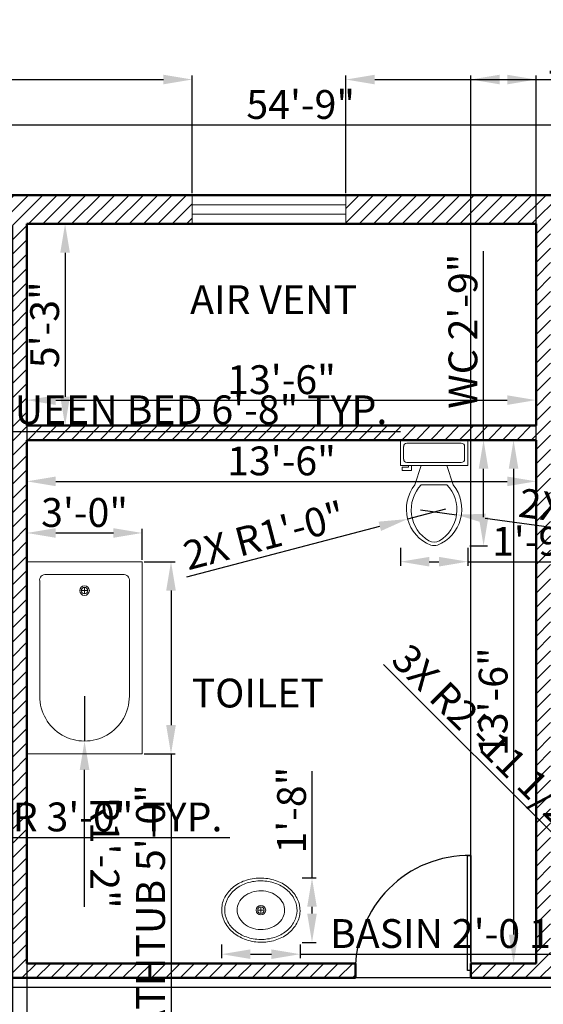
# Model space of a CAD drawing. Units: inches. Extents: x 61993 to 62774, y 55335 to 55871.
# Tile 4 of 6: x 62310 to 62474, y 55563 to 55871. Entities that reach past the tile are written whole.
import ezdxf

# ---------------------------------------------------------------- set-up
doc = ezdxf.new("R2010")
doc.units = ezdxf.units.IN
for name, color, linetype, lineweight in [('A-ANNO-DIMS', 2, 'Continuous', 18), ('A-AREA-IDEN', 7, 'Continuous', 25), ('A-DOOR', 3, 'Continuous', 25), ('A-FLOR-FIXT', 9, 'Continuous', 18), ('A-GLAZ', 4, 'Continuous', 18), ('A-WALL', 7, 'Continuous', 50)]:
    doc.layers.add(name, color=color, linetype=linetype, lineweight=lineweight)
doc.layers.add('A-WALL-PATT', color=40, linetype='Continuous', lineweight=13, true_color=0xf8d731)
doc.styles.get("Standard").update_dxf_attribs({"font": 'arial.ttf'})
doc.dimstyles.new('ISO-25', dxfattribs={"dimtxt": 9, "dimasz": 9, "dimexe": 1.25, "dimexo": 0.625, "dimtad": 1, "dimdec": 1, "dimrnd": 9, "dimlunit": 3, "dimtxsty": 'Standard', "dimcen": 2.5, "dimadec": 0, "dimazin": 0, "dimtfac": 1, "dimtdec": 1, "dimtmove": 0, "dimatfit": 3, "dimfxl": 1, "dimarcsym": 0})

# ---------------------------------------------------------------- blocks, each defined once
blk = doc.blocks.new('*D3')
at = {"layer": 'A-ANNO-DIMS', "color": 0, "lineweight": -2, "transparency": 16777216}
for p, q in [((62312.69, 55744.58), (62312.69, 55753.17)), ((62471.69, 55744.58), (62471.69, 55753.17)), ((62321.69, 55751.92), (62462.69, 55751.92))]:
    blk.add_line(p, q, dxfattribs=at)
at = {"layer": 'A-ANNO-DIMS', "color": 0, "transparency": 16777216}
for points in [[(62321.69, 55753.42), (62321.69, 55750.42), (62312.69, 55751.92)], [(62462.69, 55753.42), (62462.69, 55750.42), (62471.69, 55751.92)]]:
    blk.add_solid(points, dxfattribs=at)
at = {"layer": 'Defpoints', "color": 0, "transparency": 16777216}
for p in [(62471.69, 55751.92), (62312.69, 55743.96), (62471.69, 55743.96)]:
    blk.add_point(p, dxfattribs=at)
at = {"layer": 'A-ANNO-DIMS', "color": 0, "transparency": 16777216, "insert": (62392.19, 55757.14), "char_height": 9, "attachment_point": 5}
blk.add_mtext('13\'-6"', dxfattribs=at)
blk = doc.blocks.new('*D4')
at = {"layer": 'A-ANNO-DIMS', "color": 0, "lineweight": -2, "transparency": 16777216}
for p, q in [((62313.32, 55806.96), (62325.87, 55806.96)), ((62324.62, 55797.96), (62324.62, 55752.96)), ((62313.32, 55743.96), (62325.87, 55743.96))]:
    blk.add_line(p, q, dxfattribs=at)
at = {"layer": 'A-ANNO-DIMS', "color": 0, "transparency": 16777216}
for points in [[(62323.12, 55797.96), (62326.12, 55797.96), (62324.62, 55806.96)], [(62323.12, 55752.96), (62326.12, 55752.96), (62324.62, 55743.96)]]:
    blk.add_solid(points, dxfattribs=at)
at = {"layer": 'Defpoints', "color": 0, "transparency": 16777216}
for p in [(62312.69, 55806.96), (62312.69, 55743.96), (62324.62, 55743.96)]:
    blk.add_point(p, dxfattribs=at)
at = {"layer": 'A-ANNO-DIMS', "color": 0, "transparency": 16777216, "insert": (62319.39, 55775.46), "char_height": 9, "attachment_point": 5, "rotation": 90}
blk.add_mtext('5\'-3"', dxfattribs=at)
blk = doc.blocks.new('*D5')
at = {"layer": 'A-ANNO-DIMS', "color": 0, "lineweight": -2, "transparency": 16777216}
for p, q in [((62471.07, 55739.46), (62463.41, 55739.46)), ((62464.66, 55730.46), (62464.66, 55584.96)), ((62471.07, 55575.96), (62463.41, 55575.96))]:
    blk.add_line(p, q, dxfattribs=at)
at = {"layer": 'A-ANNO-DIMS', "color": 0, "transparency": 16777216}
for points in [[(62463.16, 55730.46), (62466.16, 55730.46), (62464.66, 55739.46)], [(62463.16, 55584.96), (62466.16, 55584.96), (62464.66, 55575.96)]]:
    blk.add_solid(points, dxfattribs=at)
at = {"layer": 'Defpoints', "color": 0, "transparency": 16777216}
for p in [(62471.69, 55739.46), (62464.66, 55575.96), (62471.69, 55575.96)]:
    blk.add_point(p, dxfattribs=at)
at = {"layer": 'A-ANNO-DIMS', "color": 0, "transparency": 16777216, "insert": (62459.44, 55657.71), "char_height": 9, "attachment_point": 5, "rotation": 90}
blk.add_mtext('13\'-6"', dxfattribs=at)
blk = doc.blocks.new('*D6')
at = {"layer": 'A-ANNO-DIMS', "color": 0, "lineweight": -2, "transparency": 16777216}
for p, q in [((62312.69, 55738.83), (62312.69, 55725.29)), ((62471.69, 55738.83), (62471.69, 55725.29)), ((62321.69, 55726.54), (62462.69, 55726.54))]:
    blk.add_line(p, q, dxfattribs=at)
at = {"layer": 'A-ANNO-DIMS', "color": 0, "transparency": 16777216}
for points in [[(62321.69, 55728.04), (62321.69, 55725.04), (62312.69, 55726.54)], [(62462.69, 55728.04), (62462.69, 55725.04), (62471.69, 55726.54)]]:
    blk.add_solid(points, dxfattribs=at)
at = {"layer": 'Defpoints', "color": 0, "transparency": 16777216}
for p in [(62312.69, 55739.46), (62471.69, 55739.46), (62471.69, 55726.54)]:
    blk.add_point(p, dxfattribs=at)
at = {"layer": 'A-ANNO-DIMS', "color": 0, "transparency": 16777216, "insert": (62392.19, 55731.76), "char_height": 9, "attachment_point": 5}
blk.add_mtext('13\'-6"', dxfattribs=at)
blk = doc.blocks.new('Toilet - top')
for p, q in [((9.5, -6), (9.5, -2)), ((-10, -8.5), (-8, -8.5)), ((-10, -9.5), (-10, -8.5)), ((-8, -8.5), (-8, -8)), ((-7, -8), (-7, -9.5)), ((-4, -8), (-6, -14)), ((4, -8), (6, -14)), ((-7, -9.5), (-10, -9.5)), ((4, -14), (-4, -14))]:
    blk.add_line(p, q)
blk.add_lwpolyline([(10.5, -8), (10.5, 0), (-10.5, 0), (-10.5, -8)], close=True)
for points in [[(-9.5, -2), (-9.5, -6)], [(8.5, -1), (-8.5, -1)], [(-8.5, -7), (8.5, -7)]]:
    blk.add_lwpolyline(points)
for centre, radius, start, end in [((-8.62, -1.88), 0.884, 81.8699, 188.1301), ((8.62, -1.88), 0.884, 351.8699, 98.1301), ((-8.62, -6.12), 0.884, 171.8699, 278.1301), ((8.62, -6.12), 0.884, 261.8699, 8.1301), ((3.52, -21.58), 12.17, 141.4691, 247.9714), ((4.2, -21.82), 11.33, 136.3677, 238.9468), ((-3.52, -21.58), 12.17, 292.0284, 38.5307), ((-4.2, -21.82), 11.33, 301.053, 43.6321), ((0, -27.88), 4, 245.7318, 294.2682), ((0, -29), 4, 254.8605, 285.1395)]:
    blk.add_arc(centre, radius, start, end)
blk = doc.blocks.new('Sink - Oval top')
for p, q in [((-1, 0), (1, 0)), ((0, 1), (0, -1))]:
    blk.add_line(p, q)
for points in [[(-12.23, 0.39, 0.117634), (-11.46, -3.36, 0.104469), (-8.88, -6.8, 0.090016), (-5.08, -9.07, 0.08192), (-0.32, -10.02, 0.08192), (4.49, -9.38, 0.090016), (8.42, -7.36, 0.104469), (11.22, -4.09, 0.117634), (12.23, -0.39, 0.117634), (11.46, 3.36, 0.104469), (8.88, 6.8, 0.090016), (5.08, 9.07, 0.08192), (0.32, 10.02, 0.08192), (-4.49, 9.38, 0.090016), (-8.42, 7.36, 0.104469), (-11.22, 4.09, 0.117634)], [(-11.29, 0.16, 0.118622), (-10.52, -3.25, 0.104678), (-8.07, -6.36, 0.089562), (-4.54, -8.37, 0.081185), (-0.13, -9.15, 0.081185), (4.3, -8.49, 0.089562), (7.89, -6.58, 0.104678), (10.42, -3.55, 0.118622), (11.29, -0.16, 0.118622), (10.52, 3.25, 0.104678), (8.07, 6.36, 0.089562), (4.54, 8.37, 0.081185), (0.13, 9.15, 0.081185), (-4.3, 8.49, 0.089562), (-7.89, 6.58, 0.104678), (-10.42, 3.55, 0.118622)], [(-7.42, 0.08, 0.118283), (-6.91, -2.17, 0.104607), (-5.29, -4.21, 0.089718), (-2.97, -5.53, 0.081436), (-0.07, -6.04, 0.081436), (2.84, -5.59, 0.089718), (5.2, -4.33, 0.104607), (6.86, -2.32, 0.118283), (7.42, -0.08, 0.118283), (6.91, 2.17, 0.104607), (5.29, 4.21, 0.089718), (2.97, 5.53, 0.081436), (0.07, 6.04, 0.081436), (-2.84, 5.59, 0.089718), (-5.2, 4.33, 0.104607), (-6.86, 2.32, 0.118283)]]:
    blk.add_lwpolyline(points, format="xyb", close=True)
for radius in [1.5, 1]:
    blk.add_circle((0, 0), radius)
blk = doc.blocks.new('Bath Tub - 26 x 60 in.')
for p, q in [((8, -18), (10, -18)), ((9, -17), (9, -19))]:
    blk.add_line(p, q)
blk.add_lwpolyline([(0, -36), (0, 0), (60, 0), (60, -36)], close=True)
for points in [[(4, -30), (4, -6)], [(6, -4), (42, -4)], [(42, -32), (6, -32)]]:
    blk.add_lwpolyline(points)
for radius in [1.5, 1]:
    blk.add_circle((9, -18), radius)
for centre, radius, start, end in [((5.75, -5.75), 1.77, 81.8699, 188.1301), ((42, -18), 14, 270, 90), ((5.75, -30.25), 1.77, 171.8699, 278.1301)]:
    blk.add_arc(centre, radius, start, end)
blk = doc.blocks.new('*D24')
at = {"layer": 'A-ANNO-DIMS', "color": 0, "lineweight": -2, "transparency": 16777216}
for p, q in [((62068.19, 55816.58), (62068.19, 55839.13)), ((62728.19, 55816.58), (62728.19, 55839.13)), ((62077.19, 55837.88), (62719.19, 55837.88))]:
    blk.add_line(p, q, dxfattribs=at)
at = {"layer": 'A-ANNO-DIMS', "color": 0, "transparency": 16777216}
for points in [[(62077.19, 55839.38), (62077.19, 55836.38), (62068.19, 55837.88)], [(62719.19, 55839.38), (62719.19, 55836.38), (62728.19, 55837.88)]]:
    blk.add_solid(points, dxfattribs=at)
at = {"layer": 'Defpoints', "color": 0, "transparency": 16777216}
for p in [(62728.19, 55837.88), (62068.19, 55815.96), (62728.19, 55815.96)]:
    blk.add_point(p, dxfattribs=at)
at = {"layer": 'A-ANNO-DIMS', "color": 0, "transparency": 16777216, "insert": (62398.19, 55843.1), "char_height": 9, "attachment_point": 5}
blk.add_mtext('54\'-9"', dxfattribs=at)
blk = doc.blocks.new('WIN-48IN')
for p, q in [((0, 9), (0, 0)), ((48, 9), (48, 0)), ((48, 6), (0, 6)), ((48, 3), (0, 3))]:
    blk.add_line(p, q)
blk = doc.blocks.new('DOOR-SINGLE-36IN')
for p, q in [((35, 0), (35, 36)), ((35, 36), (36, 36)), ((36, 36), (36, 2.25)), ((36, 0), (35, 0))]:
    blk.add_line(p, q)
blk.add_arc((35.5, 0.5), 35.5, 89.1931, 180.8069)
blk = doc.blocks.new('*D34')
at = {"layer": 'A-ANNO-DIMS', "color": 0, "lineweight": -2, "transparency": 16777216}
for p, q in [((62234.09, 55610.47), (62234.09, 55616.51)), ((62243.09, 55615.26), (62261.23, 55615.26)), ((62270.23, 55610.47), (62270.23, 55616.51)), ((62270.23, 55615.26), (62376.1, 55615.26))]:
    blk.add_line(p, q, dxfattribs=at)
at = {"layer": 'A-ANNO-DIMS', "color": 0, "transparency": 16777216}
for points in [[(62243.09, 55616.76), (62243.09, 55613.76), (62234.09, 55615.26)], [(62261.23, 55616.76), (62261.23, 55613.76), (62270.23, 55615.26)]]:
    blk.add_solid(points, dxfattribs=at)
at = {"layer": 'Defpoints', "color": 0, "transparency": 16777216}
for p in [(62270.23, 55615.26), (62234.09, 55609.84), (62270.23, 55609.84)]:
    blk.add_point(p, dxfattribs=at)
at = {"layer": 'A-ANNO-DIMS', "color": 0, "transparency": 16777216, "insert": (62327.67, 55620.55), "char_height": 9, "attachment_point": 5}
blk.add_mtext('DOOR 3\'-0" TYP.', dxfattribs=at)
blk = doc.blocks.new('*D38')
at = {"layer": 'A-ANNO-DIMS', "color": 0, "lineweight": -2, "transparency": 16777216}
for p, q in [((62206.68, 55730.79), (62206.68, 55743.42)), ((62286.68, 55730.79), (62286.68, 55743.42)), ((62215.68, 55742.17), (62277.68, 55742.17)), ((62286.68, 55742.17), (62429.32, 55742.17))]:
    blk.add_line(p, q, dxfattribs=at)
at = {"layer": 'A-ANNO-DIMS', "color": 0, "transparency": 16777216}
for points in [[(62215.68, 55743.67), (62215.68, 55740.67), (62206.68, 55742.17)], [(62277.68, 55743.67), (62277.68, 55740.67), (62286.68, 55742.17)]]:
    blk.add_solid(points, dxfattribs=at)
at = {"layer": 'Defpoints', "color": 0, "transparency": 16777216}
for p in [(62286.68, 55742.17), (62206.68, 55730.17), (62286.68, 55730.17)]:
    blk.add_point(p, dxfattribs=at)
at = {"layer": 'A-ANNO-DIMS', "color": 0, "transparency": 16777216, "insert": (62362.5, 55747.72), "char_height": 9, "attachment_point": 5}
blk.add_mtext('QUEEN BED 6\'-8" TYP.', dxfattribs=at)
blk = doc.blocks.new('*D44')
at = {"layer": 'A-ANNO-DIMS', "color": 0, "lineweight": -2, "transparency": 16777216}
for p, q in [((62455.29, 55739.46), (62455.29, 55798.44)), ((62450.96, 55739.46), (62456.54, 55739.46)), ((62455.29, 55715.41), (62455.29, 55730.46)), ((62450.96, 55706.41), (62456.54, 55706.41))]:
    blk.add_line(p, q, dxfattribs=at)
at = {"layer": 'A-ANNO-DIMS', "color": 0, "transparency": 16777216}
for points in [[(62453.79, 55730.46), (62456.79, 55730.46), (62455.29, 55739.46)], [(62453.79, 55715.41), (62456.79, 55715.41), (62455.29, 55706.41)]]:
    blk.add_solid(points, dxfattribs=at)
at = {"layer": 'Defpoints', "color": 0, "transparency": 16777216}
for p in [(62450.34, 55739.46), (62455.29, 55739.46), (62450.34, 55706.41)]:
    blk.add_point(p, dxfattribs=at)
at = {"layer": 'A-ANNO-DIMS', "color": 0, "transparency": 16777216, "insert": (62450.01, 55773.45), "char_height": 9, "attachment_point": 5, "rotation": 90}
blk.add_mtext('WC 2\'-9"', dxfattribs=at)
blk = doc.blocks.new('*D45')
at = {"layer": 'A-ANNO-DIMS', "color": 0, "lineweight": -2, "transparency": 16777216}
for p, q in [((62429.34, 55705.79), (62429.34, 55700.2)), ((62450.34, 55705.79), (62450.34, 55700.2)), ((62438.34, 55701.45), (62441.34, 55701.45)), ((62450.34, 55701.45), (62483.66, 55701.45))]:
    blk.add_line(p, q, dxfattribs=at)
at = {"layer": 'A-ANNO-DIMS', "color": 0, "transparency": 16777216}
for points in [[(62438.34, 55702.95), (62438.34, 55699.95), (62429.34, 55701.45)], [(62441.34, 55702.95), (62441.34, 55699.95), (62450.34, 55701.45)]]:
    blk.add_solid(points, dxfattribs=at)
at = {"layer": 'Defpoints', "color": 0, "transparency": 16777216}
for p in [(62429.34, 55706.41), (62450.34, 55706.41), (62450.34, 55701.45)]:
    blk.add_point(p, dxfattribs=at)
at = {"layer": 'A-ANNO-DIMS', "color": 0, "transparency": 16777216, "insert": (62471.5, 55706.67), "char_height": 9, "attachment_point": 5}
blk.add_mtext('1\'-9"', dxfattribs=at)
blk = doc.blocks.new('*D46')
at = {"layer": 'A-ANNO-DIMS', "color": 0, "lineweight": -2, "transparency": 16777216}
for p, q in [((62373.49, 55581.91), (62373.49, 55577.6)), ((62398.04, 55581.91), (62398.04, 55577.6)), ((62382.49, 55578.85), (62389.04, 55578.85)), ((62398.04, 55578.85), (62494.01, 55578.85))]:
    blk.add_line(p, q, dxfattribs=at)
at = {"layer": 'A-ANNO-DIMS', "color": 0, "transparency": 16777216}
for points in [[(62382.49, 55580.35), (62382.49, 55577.35), (62373.49, 55578.85)], [(62389.04, 55580.35), (62389.04, 55577.35), (62398.04, 55578.85)]]:
    blk.add_solid(points, dxfattribs=at)
at = {"layer": 'Defpoints', "color": 0, "transparency": 16777216}
for p in [(62373.49, 55582.54), (62398.04, 55582.54), (62398.04, 55578.85)]:
    blk.add_point(p, dxfattribs=at)
at = {"layer": 'A-ANNO-DIMS', "color": 0, "transparency": 16777216, "insert": (62450.52, 55584.13), "char_height": 9, "attachment_point": 5}
blk.add_mtext('BASIN 2\'-0 1/2"', dxfattribs=at)
blk = doc.blocks.new('*D47')
at = {"layer": 'A-ANNO-DIMS', "color": 0, "lineweight": -2, "transparency": 16777216}
for p, q in [((62401.72, 55602.67), (62401.72, 55636)), ((62398.66, 55602.67), (62402.97, 55602.67)), ((62401.72, 55591.54), (62401.72, 55593.67)), ((62398.66, 55582.54), (62402.97, 55582.54))]:
    blk.add_line(p, q, dxfattribs=at)
at = {"layer": 'A-ANNO-DIMS', "color": 0, "transparency": 16777216}
for points in [[(62400.22, 55593.67), (62403.22, 55593.67), (62401.72, 55602.67)], [(62400.22, 55591.54), (62403.22, 55591.54), (62401.72, 55582.54)]]:
    blk.add_solid(points, dxfattribs=at)
at = {"layer": 'Defpoints', "color": 0, "transparency": 16777216}
for p in [(62398.04, 55602.67), (62401.72, 55602.67), (62398.04, 55582.54)]:
    blk.add_point(p, dxfattribs=at)
at = {"layer": 'A-ANNO-DIMS', "color": 0, "transparency": 16777216, "insert": (62396.5, 55623.84), "char_height": 9, "attachment_point": 5, "rotation": 90}
blk.add_mtext('1\'-8"', dxfattribs=at)
blk = doc.blocks.new('*D48')
at = {"layer": 'A-ANNO-DIMS', "color": 0, "lineweight": -2, "transparency": 16777216}
for p, q in [((62349.32, 55701.42), (62358.94, 55701.42)), ((62357.69, 55692.42), (62357.69, 55650.42)), ((62349.32, 55641.42), (62358.94, 55641.42)), ((62357.69, 55641.42), (62357.69, 55545.48))]:
    blk.add_line(p, q, dxfattribs=at)
at = {"layer": 'A-ANNO-DIMS', "color": 0, "transparency": 16777216}
for points in [[(62356.19, 55692.42), (62359.19, 55692.42), (62357.69, 55701.42)], [(62356.19, 55650.42), (62359.19, 55650.42), (62357.69, 55641.42)]]:
    blk.add_solid(points, dxfattribs=at)
at = {"layer": 'Defpoints', "color": 0, "transparency": 16777216}
for p in [(62348.69, 55701.42), (62348.69, 55641.42), (62357.69, 55641.42)]:
    blk.add_point(p, dxfattribs=at)
at = {"layer": 'A-ANNO-DIMS', "color": 0, "transparency": 16777216, "insert": (62352.47, 55588.95), "char_height": 9, "attachment_point": 5, "rotation": 90}
blk.add_mtext('BATHTUB 5\'-0"', dxfattribs=at)
blk = doc.blocks.new('*D49')
at = {"layer": 'A-ANNO-DIMS', "color": 0, "lineweight": -2, "transparency": 16777216}
for p, q in [((62312.69, 55702.05), (62312.69, 55711.67)), ((62321.69, 55710.42), (62339.69, 55710.42)), ((62348.69, 55702.05), (62348.69, 55711.67))]:
    blk.add_line(p, q, dxfattribs=at)
at = {"layer": 'A-ANNO-DIMS', "color": 0, "transparency": 16777216}
for points in [[(62321.69, 55711.92), (62321.69, 55708.92), (62312.69, 55710.42)], [(62339.69, 55711.92), (62339.69, 55708.92), (62348.69, 55710.42)]]:
    blk.add_solid(points, dxfattribs=at)
at = {"layer": 'Defpoints', "color": 0, "transparency": 16777216}
for p in [(62348.69, 55710.42), (62312.69, 55701.42), (62348.69, 55701.42)]:
    blk.add_point(p, dxfattribs=at)
at = {"layer": 'A-ANNO-DIMS', "color": 0, "transparency": 16777216, "insert": (62330.69, 55715.65), "char_height": 9, "attachment_point": 5}
blk.add_mtext('3\'-0"', dxfattribs=at)
blk = doc.blocks.new('*D65')
at = {"layer": 'A-ANNO-DIMS', "color": 0, "lineweight": -2, "transparency": 16777216}
for p, q in [((62186.51, 55816.58), (62186.51, 55853.31)), ((62195.51, 55852.06), (62355.31, 55852.06)), ((62364.31, 55816.58), (62364.31, 55853.31))]:
    blk.add_line(p, q, dxfattribs=at)
at = {"layer": 'A-ANNO-DIMS', "color": 0, "transparency": 16777216}
for points in [[(62195.51, 55853.56), (62195.51, 55850.56), (62186.51, 55852.06)], [(62355.31, 55853.56), (62355.31, 55850.56), (62364.31, 55852.06)]]:
    blk.add_solid(points, dxfattribs=at)
at = {"layer": 'Defpoints', "color": 0, "transparency": 16777216}
for p in [(62364.31, 55852.06), (62186.51, 55815.96), (62364.31, 55815.96)]:
    blk.add_point(p, dxfattribs=at)
at = {"layer": 'A-ANNO-DIMS', "color": 0, "transparency": 16777216, "insert": (62275.41, 55857.28), "char_height": 9, "attachment_point": 5}
blk.add_mtext('14\'-10"', dxfattribs=at)
blk = doc.blocks.new('*D66')
at = {"layer": 'A-ANNO-DIMS', "color": 0, "lineweight": -2, "transparency": 16777216}
for p, q in [((62412.31, 55816.58), (62412.31, 55853.31)), ((62421.31, 55852.06), (62569.07, 55852.06)), ((62578.07, 55816.58), (62578.07, 55853.31))]:
    blk.add_line(p, q, dxfattribs=at)
at = {"layer": 'A-ANNO-DIMS', "color": 0, "transparency": 16777216}
for points in [[(62421.31, 55853.56), (62421.31, 55850.56), (62412.31, 55852.06)], [(62569.07, 55853.56), (62569.07, 55850.56), (62578.07, 55852.06)]]:
    blk.add_solid(points, dxfattribs=at)
at = {"layer": 'Defpoints', "color": 0, "transparency": 16777216}
for p in [(62578.07, 55852.06), (62412.31, 55815.96), (62578.07, 55815.96)]:
    blk.add_point(p, dxfattribs=at)
at = {"layer": 'A-ANNO-DIMS', "color": 0, "transparency": 16777216, "insert": (62495.19, 55857.28), "char_height": 9, "attachment_point": 5}
blk.add_mtext('13\'-10"', dxfattribs=at)
blk = doc.blocks.new('*D72')
at = {"layer": 'A-ANNO-DIMS', "color": 0, "lineweight": -2, "transparency": 16777216}
for p, q in [((62451.32, 55576.58), (62451.32, 55853.31)), ((62460.32, 55852.06), (62462.69, 55852.06)), ((62471.69, 55576.58), (62471.69, 55853.31)), ((62471.69, 55852.06), (62525.99, 55852.06))]:
    blk.add_line(p, q, dxfattribs=at)
at = {"layer": 'A-ANNO-DIMS', "color": 0, "transparency": 16777216}
for points in [[(62460.32, 55853.56), (62460.32, 55850.56), (62451.32, 55852.06)], [(62462.69, 55853.56), (62462.69, 55850.56), (62471.69, 55852.06)]]:
    blk.add_solid(points, dxfattribs=at)
at = {"layer": 'Defpoints', "color": 0, "transparency": 16777216}
for p in [(62471.69, 55852.06), (62451.32, 55575.96), (62471.69, 55575.96)]:
    blk.add_point(p, dxfattribs=at)
at = {"layer": 'A-ANNO-DIMS', "color": 0, "transparency": 16777216, "insert": (62503.34, 55857.33), "char_height": 9, "attachment_point": 5}
blk.add_mtext('1\'-8 1/2"', dxfattribs=at)
blk = doc.blocks.new('*D74')
at = {"layer": 'A-ANNO-DIMS', "color": 0, "lineweight": -2, "transparency": 16777216}
for p, q in [((62032.09, 55580.46), (62032.09, 55589.46)), ((62547.57, 55571.46), (62030.84, 55571.46)), ((62032.09, 55571.46), (62032.09, 55568.46)), ((62547.57, 55568.46), (62030.84, 55568.46)), ((62032.09, 55559.46), (62032.09, 55525.28))]:
    blk.add_line(p, q, dxfattribs=at)
at = {"layer": 'A-ANNO-DIMS', "color": 0, "transparency": 16777216}
for points in [[(62030.59, 55580.46), (62033.59, 55580.46), (62032.09, 55571.46)], [(62030.59, 55559.46), (62033.59, 55559.46), (62032.09, 55568.46)]]:
    blk.add_solid(points, dxfattribs=at)
at = {"layer": 'Defpoints', "color": 0, "transparency": 16777216}
for p in [(62548.19, 55571.46), (62032.09, 55568.46), (62548.19, 55568.46)]:
    blk.add_point(p, dxfattribs=at)
at = {"layer": 'A-ANNO-DIMS', "color": 0, "transparency": 16777216, "insert": (62026.87, 55537.87), "char_height": 9, "attachment_point": 5, "rotation": 90}
blk.add_mtext('0\'-3"', dxfattribs=at)
blk = doc.blocks.new('*D75')
at = {"layer": 'A-ANNO-DIMS', "color": 0, "lineweight": -2, "transparency": 16777216}
for p, q in [((62308.19, 55806.33), (62308.19, 55358.61)), ((62312.69, 55806.33), (62312.69, 55358.61)), ((62299.19, 55359.86), (62290.19, 55359.86)), ((62308.19, 55359.86), (62312.69, 55359.86)), ((62321.69, 55359.86), (62376.84, 55359.86))]:
    blk.add_line(p, q, dxfattribs=at)
at = {"layer": 'A-ANNO-DIMS', "color": 0, "transparency": 16777216}
for points in [[(62299.19, 55361.36), (62299.19, 55358.36), (62308.19, 55359.86)], [(62321.69, 55361.36), (62321.69, 55358.36), (62312.69, 55359.86)]]:
    blk.add_solid(points, dxfattribs=at)
at = {"layer": 'Defpoints', "color": 0, "transparency": 16777216}
for p in [(62308.19, 55806.96), (62312.69, 55806.96), (62312.69, 55359.86)]:
    blk.add_point(p, dxfattribs=at)
at = {"layer": 'A-ANNO-DIMS', "color": 0, "transparency": 16777216, "insert": (62353.77, 55365.13), "char_height": 9, "attachment_point": 5}
blk.add_mtext('0\'-4 1/2"', dxfattribs=at)
blk = doc.blocks.new('*D87')
at = {"layer": 'A-ANNO-DIMS', "color": 0, "lineweight": -2, "transparency": 16777216}
for p, q in [((62424.07, 55669.37), (62487.77, 55605.68)), ((62519.24, 55574.21), (62494.13, 55599.31))]:
    blk.add_line(p, q, dxfattribs=at)
at = {"layer": 'A-ANNO-DIMS', "color": 0, "transparency": 16777216}
blk.add_solid([(62488.83, 55606.74), (62486.71, 55604.61), (62494.13, 55599.31)], dxfattribs=at)
at = {"layer": 'Defpoints', "color": 0, "transparency": 16777216}
for p in [(62494.13, 55599.31), (62519.24, 55574.21)]:
    blk.add_point(p, dxfattribs=at)
at = {"layer": 'A-ANNO-DIMS', "color": 0, "transparency": 16777216, "insert": (62456.47, 55644.44), "char_height": 9, "attachment_point": 5, "rotation": 315}
blk.add_mtext('3X R2\'-11 1/2"', dxfattribs=at)
blk = doc.blocks.new('*D88')
at = {"layer": 'A-ANNO-DIMS', "color": 0, "lineweight": -2, "transparency": 16777216}
for p, q in [((62330.69, 55659.42), (62330.69, 55645.42)), ((62330.7, 55593.64), (62330.7, 55636.42))]:
    blk.add_line(p, q, dxfattribs=at)
at = {"layer": 'A-ANNO-DIMS', "color": 0, "transparency": 16777216}
blk.add_solid([(62332.2, 55636.42), (62329.2, 55636.42), (62330.69, 55645.42)], dxfattribs=at)
at = {"layer": 'Defpoints', "color": 0, "transparency": 16777216}
for p in [(62330.69, 55659.42), (62330.69, 55645.42)]:
    blk.add_point(p, dxfattribs=at)
at = {"layer": 'A-ANNO-DIMS', "color": 0, "transparency": 16777216, "insert": (62335.84, 55610.53), "char_height": 9, "attachment_point": 5, "rotation": 270.002}
blk.add_mtext('R1\'-2"', dxfattribs=at)
blk = doc.blocks.new('*D89')
at = {"layer": 'A-ANNO-DIMS', "color": 0, "lineweight": -2, "transparency": 16777216}
for p, q in [((62443.36, 55717.88), (62431.59, 55714.78)), ((62362.65, 55696.67), (62422.88, 55712.5))]:
    blk.add_line(p, q, dxfattribs=at)
at = {"layer": 'A-ANNO-DIMS', "color": 0, "transparency": 16777216}
blk.add_solid([(62422.5, 55713.95), (62423.26, 55711.05), (62431.59, 55714.78)], dxfattribs=at)
at = {"layer": 'Defpoints', "color": 0, "transparency": 16777216}
for p in [(62443.36, 55717.88), (62431.59, 55714.78)]:
    blk.add_point(p, dxfattribs=at)
at = {"layer": 'A-ANNO-DIMS', "color": 0, "transparency": 16777216, "insert": (62387.09, 55708.49), "char_height": 9, "attachment_point": 5, "rotation": 14.719}
blk.add_mtext('2X R1\'-0"', dxfattribs=at)
blk = doc.blocks.new('*D90')
at = {"layer": 'A-ANNO-DIMS', "color": 0, "lineweight": -2, "transparency": 16777216}
for p, q in [((62435.64, 55717.64), (62446.86, 55716.13)), ((62545.22, 55702.9), (62455.78, 55714.93))]:
    blk.add_line(p, q, dxfattribs=at)
at = {"layer": 'A-ANNO-DIMS', "color": 0, "transparency": 16777216}
blk.add_solid([(62455.98, 55716.42), (62455.58, 55713.44), (62446.86, 55716.13)], dxfattribs=at)
at = {"layer": 'Defpoints', "color": 0, "transparency": 16777216}
for p in [(62435.64, 55717.64), (62446.86, 55716.13)]:
    blk.add_point(p, dxfattribs=at)
at = {"layer": 'A-ANNO-DIMS', "color": 0, "transparency": 16777216, "insert": (62505.67, 55713.55), "char_height": 9, "attachment_point": 5, "rotation": 352.3402}
blk.add_mtext('2X R0\'-11 1/2"', dxfattribs=at)

msp = doc.modelspace()

# ---------------------------------------------------------------- hatches: boundary and pattern name
at = {"layer": 'A-WALL-PATT'}
h = msp.add_hatch(dxfattribs=at)
h.set_pattern_fill('ANSI31', color=256)
h.paths.add_polyline_path([(62077.19, 55665.16), (62068.19, 55665.16), (62068.19, 55518.96), (62077.19, 55518.96), (62077.19, 55571.46), (62234.23, 55571.46), (62234.23, 55573.71, -0.007042), (62234.23, 55574.71), (62234.23, 55575.96), (62077.19, 55575.96)])
h.paths.add_polyline_path([(62077.19, 55806.96), (62138.51, 55806.96), (62138.51, 55815.96), (62068.19, 55815.96), (62068.19, 55713.16), (62077.19, 55713.16)])
h.paths.add_polyline_path([(62364.31, 55815.96), (62186.51, 55815.96), (62186.51, 55806.96), (62308.19, 55806.96), (62308.19, 55575.96), (62270.23, 55575.96), (62270.23, 55571.46), (62415.32, 55571.46), (62415.32, 55573.71, -0.007042), (62415.32, 55574.71), (62415.32, 55575.96), (62312.69, 55575.96), (62312.69, 55739.46), (62471.69, 55739.46), (62471.69, 55575.96), (62451.32, 55575.96), (62451.32, 55571.46), (62483.74, 55571.46), (62483.74, 55573.71, -0.007042), (62483.74, 55574.71), (62483.74, 55575.96), (62476.19, 55575.96), (62476.19, 55806.96), (62578.07, 55806.96), (62578.07, 55815.96), (62412.31, 55815.96), (62412.31, 55806.96), (62471.69, 55806.96), (62471.69, 55743.96), (62312.69, 55743.96), (62312.69, 55806.96), (62364.31, 55806.96)])
h.paths.add_polyline_path([(62728.19, 55815.96), (62626.07, 55815.96), (62626.07, 55806.96), (62719.19, 55806.96), (62719.19, 55739.46), (62728.19, 55739.46)])
h.paths.add_polyline_path([(62728.19, 55691.46), (62719.19, 55691.46), (62719.19, 55575.96), (62519.74, 55575.96), (62519.74, 55571.46), (62543.69, 55571.46), (62543.69, 55568.46), (62548.19, 55568.46), (62548.19, 55571.46), (62719.19, 55571.46), (62719.19, 55517.72), (62728.19, 55517.72)])
h.paths.add_polyline_path([(62599.31, 55404.96), (62548.19, 55404.96), (62548.19, 55532.46), (62546.94, 55532.46, -0.007042), (62545.94, 55532.46), (62543.69, 55532.46), (62543.69, 55404.96), (62444.22, 55404.96), (62444.22, 55395.96), (62599.31, 55395.96)])
h.paths.add_polyline_path([(62728.19, 55469.72), (62719.19, 55469.72), (62719.19, 55404.96), (62647.31, 55404.96), (62647.31, 55395.96), (62728.19, 55395.96)])
h.paths.add_polyline_path([(62396.22, 55404.96), (62309.17, 55404.96), (62309.17, 55395.96), (62396.22, 55395.96)])
h.paths.add_polyline_path([(62213.17, 55404.96), (62077.19, 55404.96), (62077.19, 55470.96), (62068.19, 55470.96), (62068.19, 55395.96), (62213.17, 55395.96)])

# ---------------------------------------------------------------- linework, layer by layer
at = {"layer": 'A-WALL'}
for p, q in [((62728.19, 55815.96), (62068.19, 55815.96)), ((62312.69, 55806.96), (62312.69, 55743.96)), ((62471.69, 55806.96), (62312.69, 55806.96)), ((62471.69, 55806.96), (62471.69, 55743.96)), ((62471.69, 55743.96), (62312.69, 55743.96)), ((62471.69, 55739.46), (62312.69, 55739.46)), ((62312.69, 55739.46), (62312.69, 55575.96)), ((62471.69, 55739.46), (62471.69, 55575.96)), ((62415.32, 55575.96), (62312.69, 55575.96)), ((62415.32, 55575.96), (62415.32, 55571.46)), ((62471.69, 55575.96), (62451.32, 55575.96)), ((62451.32, 55575.96), (62451.32, 55571.46)), ((62415.32, 55571.46), (62270.23, 55571.46)), ((62483.74, 55571.46), (62451.32, 55571.46))]:
    msp.add_line(p, q, dxfattribs=at)

# ---------------------------------------------------------------- block references
at = {"layer": 'A-DOOR'}
msp.add_blockref('DOOR-SINGLE-36IN', (62415.32, 55573.71), dxfattribs=at)
at = {"layer": 'A-FLOR-FIXT'}
for name, p in [('Toilet - top', (62439.84, 55739.46)), ('Sink - Oval top', (62385.76, 55592.6))]:
    msp.add_blockref(name, p, dxfattribs=at)
at = {"layer": 'A-FLOR-FIXT', "rotation": 270}
msp.add_blockref('Bath Tub - 26 x 60 in.', (62348.69, 55701.42), dxfattribs=at)
at = {"layer": 'A-GLAZ'}
msp.add_blockref('WIN-48IN', (62364.31, 55806.96), dxfattribs=at)

# ---------------------------------------------------------------- texts
at = {"layer": 'A-AREA-IDEN', "char_height": 9, "attachment_point": 1}
for s, insert in [('AIR VENT', (62363.66, 55787.81)), ('TOILET', (62364.13, 55664.91))]:
    msp.add_mtext_dynamic_manual_height_columns(s, width=116.6414, gutter_width=12.5, heights=[0], dxfattribs=dict(at, insert=insert))

# ---------------------------------------------------------------- dimensions: what is measured, and where the dimension line sits
at = {"layer": 'A-ANNO-DIMS'}
for base, p1, p2, override, picture, middle in [((62471.69, 55852.06), (62451.32, 55575.96), (62471.69, 55575.96), {"dimdec": 1, "dimlfac": 1, "dimrnd": 0, "dimzin": 1, "dimdsep": 46, "dimlunit": 4, "dimfrac": 2}, '*D72', (62503.34, 55857.33)), ((62364.31, 55852.06), (62186.51, 55815.96), (62364.31, 55815.96), {"dimdec": 1, "dimlfac": 1, "dimrnd": 0, "dimzin": 1, "dimdsep": 46, "dimlunit": 4, "dimfrac": 2}, '*D65', (62275.41, 55857.28)), ((62578.07, 55852.06), (62412.31, 55815.96), (62578.07, 55815.96), {"dimdec": 1, "dimlfac": 1, "dimrnd": 0, "dimzin": 1, "dimdsep": 46, "dimlunit": 4, "dimfrac": 2}, '*D66', (62495.19, 55857.28)), ((62728.19, 55837.88), (62068.19, 55815.96), (62728.19, 55815.96), {"dimclrd": 0, "dimclre": 0, "dimclrt": 0}, '*D24', (62398.19, 55843.1)), ((62312.69, 55359.86), (62308.19, 55806.96), (62312.69, 55806.96), {"dimdec": 1, "dimlfac": 1, "dimrnd": 0, "dimzin": 1, "dimdsep": 46, "dimlunit": 4, "dimfrac": 2}, '*D75', (62353.77, 55365.13)), ((62471.69, 55751.92), (62312.69, 55743.96), (62471.69, 55743.96), {"dimclrd": 0, "dimclre": 0, "dimclrt": 0}, '*D3', (62392.19, 55757.14)), ((62471.69, 55726.54), (62312.69, 55739.46), (62471.69, 55739.46), {"dimclrd": 0, "dimclre": 0, "dimclrt": 0}, '*D6', (62392.19, 55731.76)), ((62348.69, 55710.42), (62312.69, 55701.42), (62348.69, 55701.42), {"dimdec": 1, "dimlfac": 1, "dimrnd": 0, "dimzin": 1, "dimdsep": 46, "dimlunit": 4, "dimfrac": 2}, '*D49', (62330.69, 55715.65)), ((62450.34, 55701.45), (62429.34, 55706.41), (62450.34, 55706.41), {"dimdec": 1, "dimlfac": 1, "dimrnd": 0, "dimzin": 1, "dimdsep": 46, "dimlunit": 4, "dimfrac": 2}, '*D45', (62471.5, 55706.67))]:
    dim = msp.add_linear_dim(base=base, p1=p1, p2=p2, dimstyle='ISO-25', override=override, dxfattribs=at)
    dim.commit()
    dim.dimension.update_dxf_attribs({"geometry": picture, "text_midpoint": middle})
for base, p1, p2, override, picture, middle in [((62324.62, 55743.96), (62312.69, 55806.96), (62312.69, 55743.96), {"dimclrd": 0, "dimclre": 0, "dimclrt": 0}, '*D4', (62319.39, 55775.46)), ((62464.66, 55575.96), (62471.69, 55739.46), (62471.69, 55575.96), {"dimclrd": 0, "dimclre": 0, "dimclrt": 0}, '*D5', (62459.44, 55657.71)), ((62401.72, 55602.67), (62398.04, 55582.54), (62398.04, 55602.67), {"dimdec": 1, "dimlfac": 1, "dimrnd": 0, "dimzin": 1, "dimdsep": 46, "dimlunit": 4, "dimfrac": 2}, '*D47', (62396.5, 55623.84)), ((62032.09, 55568.46), (62548.19, 55571.46), (62548.19, 55568.46), {"dimdec": 1, "dimlfac": 1, "dimrnd": 0, "dimzin": 1, "dimdsep": 46, "dimlunit": 4, "dimfrac": 2}, '*D74', (62026.87, 55537.87))]:
    dim = msp.add_linear_dim(base=base, p1=p1, p2=p2, angle=90, dimstyle='ISO-25', override=override, dxfattribs=at)
    dim.commit()
    dim.dimension.update_dxf_attribs({"geometry": picture, "text_midpoint": middle})
for base, p1, p2, angle, text, picture, middle in [((62455.2935, 55739.4565), (62450.3365, 55706.4103), (62450.3365, 55739.4565), 90, 'WC <>', '*D44', (62450.015, 55773.4478)), ((62357.69, 55641.42), (62348.69, 55701.42), (62348.69, 55641.42), 270, 'BATHTUB <>', '*D48', (62352.47, 55588.95))]:
    dim = msp.add_linear_dim(base=base, p1=p1, p2=p2, angle=angle, text=text, dimstyle='ISO-25', override={"dimdec": 1, "dimlfac": 1, "dimrnd": 0, "dimzin": 1, "dimdsep": 46, "dimlunit": 4, "dimfrac": 2}, dxfattribs=at)
    dim.commit()
    dim.dimension.update_dxf_attribs({"geometry": picture, "text_midpoint": middle})
for base, p1, p2, text, picture, middle in [((62286.68, 55742.17), (62206.68, 55730.17), (62286.68, 55730.17), 'QUEEN BED <> TYP.', '*D38', (62362.5, 55747.72)), ((62270.23, 55615.26), (62234.09, 55609.84), (62270.23, 55609.84), 'DOOR <> TYP.', '*D34', (62327.67, 55620.55)), ((62398.0388, 55578.8531), (62373.4879, 55582.5357), (62398.0388, 55582.5357), 'BASIN <>', '*D46', (62450.5243, 55584.1315))]:
    dim = msp.add_linear_dim(base=base, p1=p1, p2=p2, text=text, dimstyle='ISO-25', override={"dimdec": 1, "dimlfac": 1, "dimrnd": 0, "dimzin": 1, "dimdsep": 46, "dimlunit": 4, "dimfrac": 2}, dxfattribs=at)
    dim.commit()
    dim.dimension.update_dxf_attribs({"geometry": picture, "text_midpoint": middle})
for center, mpoint, text, picture, middle in [((62435.64, 55717.64), (62446.86, 55716.13), '2X <>', '*D90', (62505.67, 55713.55)), ((62443.36, 55717.88), (62431.59, 55714.78), '2X <>', '*D89', (62387.09, 55708.49)), ((62519.24, 55574.21), (62494.13, 55599.31), '3X <>', '*D87', (62456.47, 55644.44))]:
    dim = msp.add_radius_dim(center=center, mpoint=mpoint, text=text, dimstyle='ISO-25', override={"dimdec": 1, "dimlfac": 1, "dimrnd": 0, "dimzin": 1, "dimdsep": 46, "dimlunit": 4, "dimfrac": 2}, dxfattribs=at)
    dim.commit()
    dim.dimension.update_dxf_attribs({"geometry": picture, "text_midpoint": middle})
dim = msp.add_radius_dim(center=(62330.69, 55659.42), mpoint=(62330.69, 55645.42), dimstyle='ISO-25', override={"dimdec": 1, "dimlfac": 1, "dimrnd": 0, "dimzin": 1, "dimdsep": 46, "dimlunit": 4, "dimfrac": 2}, dxfattribs=at)
dim.commit()
dim.dimension.update_dxf_attribs({"geometry": '*D88', "text_midpoint": (62335.84, 55610.53)})

doc.saveas('drawing.dxf')
